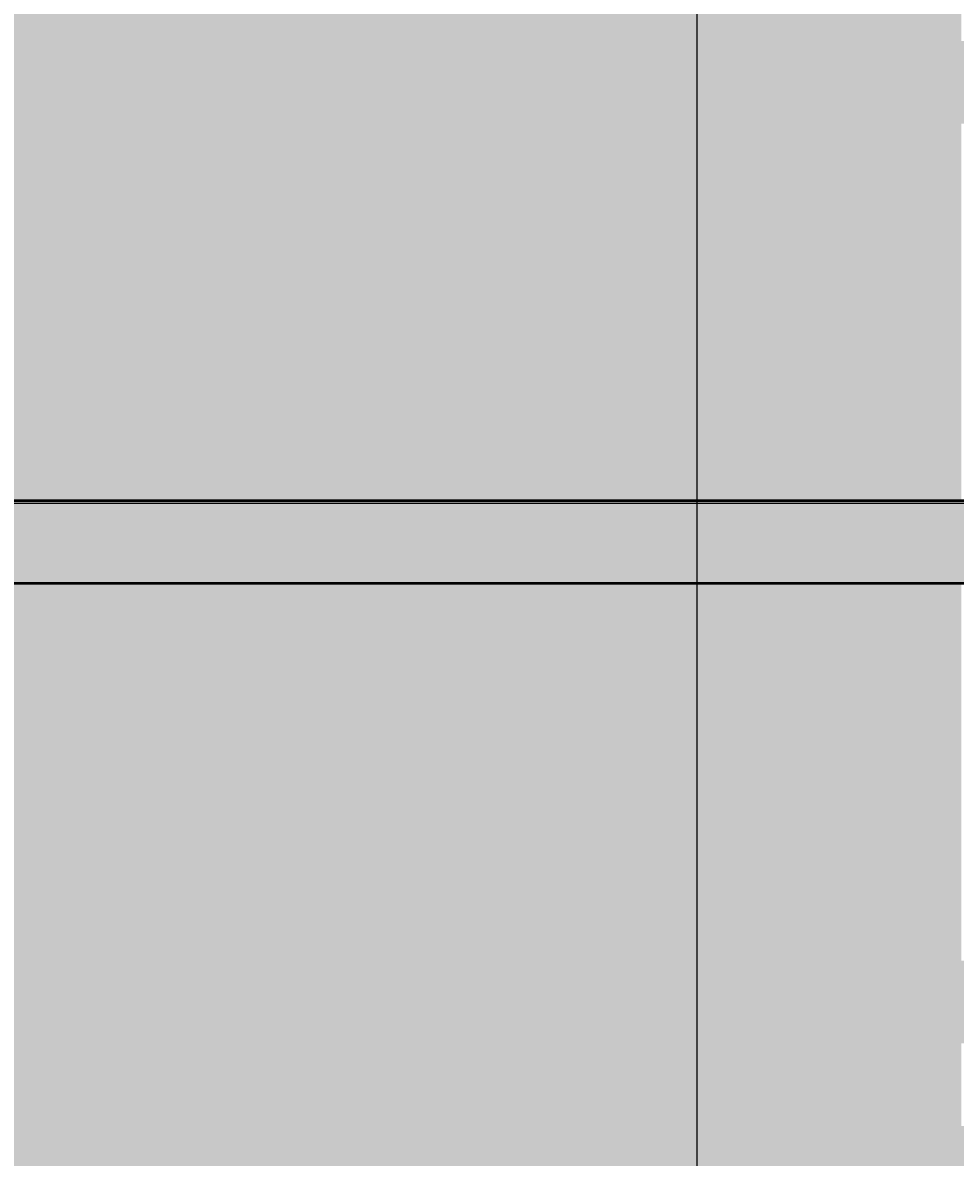
# Model space of a CAD drawing. Units: inches. Extents: x -12 to 334, y -10 to 186.
# Tile 15 of 77: x 42 to 64, y 65 to 92. Entities that reach past the tile are written whole.
import ezdxf

# ---------------------------------------------------------------- set-up
doc = ezdxf.new("R2010")
doc.units = ezdxf.units.IN
doc.header["$MEASUREMENT"] = 0
for name, color, linetype, lineweight in [('M-DIMS', 2, 'Continuous', 18), ('M-EQPM', 7, 'Continuous', 50), ('M-EQPM-PATT', 8, 'Continuous', 18)]:
    doc.layers.add(name, color=color, linetype=linetype, lineweight=lineweight)
doc.styles.get("Standard").update_dxf_attribs({"font": 'arial.ttf'})
doc.dimstyles.get("Standard").update_dxf_attribs({"dimtxt": 0.18, "dimasz": 0.18, "dimexe": 0.18, "dimexo": 0.0625, "dimgap": 0.09, "dimtad": 0, "dimtih": 1, "dimtoh": 1, "dimdec": 4, "dimzin": 0, "dimdsep": 46, "dimtxsty": 'Standard', "dimcen": 0.09, "dimadec": 0, "dimazin": 0, "dimtfac": 1, "dimtdec": 4, "dimtofl": 0, "dimtmove": 0, "dimatfit": 3, "dimfxl": 1, "dimtolj": 1, "dimtzin": 0, "dimarcsym": 0})

# ---------------------------------------------------------------- blocks, each defined once
blk = doc.blocks.new('*D1')
at = {"layer": 'Defpoints', "color": 0, "transparency": 16777216}
for p in [(281.426, 91.899), (3.376, 80.692), (281.426, 14.304)]:
    blk.add_point(p, dxfattribs=at)
at = {"layer": 'M-DIMS', "color": 0, "lineweight": -2, "transparency": 16777216}
for p, q in [((281.426, 91.836), (281.426, 14.124)), ((3.376, 80.629), (3.376, 14.124)), ((3.556, 14.304), (141.935, 14.304)), ((281.246, 14.304), (142.867, 14.304))]:
    blk.add_line(p, q, dxfattribs=at)
at = {"layer": 'M-DIMS', "color": 0, "transparency": 16777216}
for points in [[(3.556, 14.334), (3.556, 14.274), (3.376, 14.304)], [(281.246, 14.334), (281.246, 14.274), (281.426, 14.304)]]:
    blk.add_solid(points, dxfattribs=at)
at = {"layer": 'M-DIMS', "color": 0, "transparency": 16777216, "insert": (142.401, 14.304), "char_height": 0.18, "attachment_point": 5}
blk.add_mtext('\\A1;278.05', dxfattribs=at)
blk = doc.blocks.new('*D14')
at = {"layer": 'Defpoints', "color": 0, "transparency": 16777216}
for p in [(63.5, 109.058), (-11.174, 49.45), (64.207, 49.45)]:
    blk.add_point(p, dxfattribs=at)
at = {"layer": 'M-DIMS', "color": 0, "lineweight": -2, "transparency": 16777216}
for p, q in [((63.438, 109.058), (-11.354, 109.058)), ((-11.174, 108.878), (-11.174, 79.436)), ((-11.174, 49.63), (-11.174, 79.072)), ((64.144, 49.45), (-11.354, 49.45))]:
    blk.add_line(p, q, dxfattribs=at)
at = {"layer": 'M-DIMS', "color": 0, "transparency": 16777216}
for points in [[(-11.204, 108.878), (-11.144, 108.878), (-11.174, 109.058)], [(-11.204, 49.63), (-11.144, 49.63), (-11.174, 49.45)]]:
    blk.add_solid(points, dxfattribs=at)
at = {"layer": 'M-DIMS', "color": 0, "transparency": 16777216, "insert": (-11.174, 79.254), "char_height": 0.18, "attachment_point": 5}
blk.add_mtext('\\A1;59.61', dxfattribs=at)
blk = doc.blocks.new('*D26')
at = {"layer": 'Defpoints', "color": 0, "transparency": 16777216}
for p in [(87.888, 169.385), (87.888, 56.321), (58.1, 33.675)]:
    blk.add_point(p, dxfattribs=at)
at = {"layer": 'M-DIMS', "color": 0, "lineweight": -2, "transparency": 16777216}
for p, q in [((58.1, 33.738), (58.1, 169.565)), ((58.28, 169.385), (72.599, 169.385)), ((87.708, 169.385), (73.389, 169.385)), ((87.888, 56.383), (87.888, 169.565))]:
    blk.add_line(p, q, dxfattribs=at)
at = {"layer": 'M-DIMS', "color": 0, "transparency": 16777216}
for points in [[(58.28, 169.415), (58.28, 169.355), (58.1, 169.385)], [(87.708, 169.415), (87.708, 169.355), (87.888, 169.385)]]:
    blk.add_solid(points, dxfattribs=at)
at = {"layer": 'M-DIMS', "color": 0, "transparency": 16777216, "insert": (72.994, 169.385), "char_height": 0.18, "attachment_point": 5}
blk.add_mtext('\\A1;29.79', dxfattribs=at)
blk = doc.blocks.new('*D35')
at = {"layer": 'Defpoints', "color": 0, "transparency": 16777216}
for p in [(216.428, 98.108), (-11.174, 61.105), (216.428, 61.105)]:
    blk.add_point(p, dxfattribs=at)
at = {"layer": 'M-DIMS', "color": 0, "lineweight": -2, "transparency": 16777216}
for p, q in [((216.365, 98.108), (-11.354, 98.108)), ((-11.174, 97.928), (-11.174, 79.788)), ((-11.174, 61.285), (-11.174, 79.424)), ((216.365, 61.105), (-11.354, 61.105))]:
    blk.add_line(p, q, dxfattribs=at)
at = {"layer": 'M-DIMS', "color": 0, "transparency": 16777216}
for points in [[(-11.204, 97.928), (-11.144, 97.928), (-11.174, 98.108)], [(-11.204, 61.285), (-11.144, 61.285), (-11.174, 61.105)]]:
    blk.add_solid(points, dxfattribs=at)
at = {"layer": 'M-DIMS', "color": 0, "transparency": 16777216, "insert": (-11.174, 79.606), "char_height": 0.18, "attachment_point": 5}
blk.add_mtext('\\A1;37', dxfattribs=at)
blk = doc.blocks.new('*D39')
at = {"layer": 'Defpoints', "color": 0, "transparency": 16777216}
for p in [(279.726, 80.692), (-11.174, 45.854), (269.381, 45.854)]:
    blk.add_point(p, dxfattribs=at)
at = {"layer": 'M-DIMS', "color": 0, "lineweight": -2, "transparency": 16777216}
for p, q in [((279.664, 80.692), (-11.354, 80.692)), ((-11.174, 80.512), (-11.174, 63.455)), ((-11.174, 46.034), (-11.174, 63.091)), ((269.318, 45.854), (-11.354, 45.854))]:
    blk.add_line(p, q, dxfattribs=at)
at = {"layer": 'M-DIMS', "color": 0, "transparency": 16777216}
for points in [[(-11.204, 80.512), (-11.144, 80.512), (-11.174, 80.692)], [(-11.204, 46.034), (-11.144, 46.034), (-11.174, 45.854)]]:
    blk.add_solid(points, dxfattribs=at)
at = {"layer": 'M-DIMS', "color": 0, "transparency": 16777216, "insert": (-11.174, 63.273), "char_height": 0.18, "attachment_point": 5}
blk.add_mtext('\\A1;34.84', dxfattribs=at)

msp = doc.modelspace()

# ---------------------------------------------------------------- hatches: boundary and pattern name
at = {"layer": 'M-EQPM-PATT'}
h = msp.add_hatch(color=256, dxfattribs=at)
h.set_gradient(color1=(99, 100, 102), color2=(99, 100, 102), tint=1)
h.paths.add_polyline_path([(4.3766, 80.754, -0.4132606), (23.5807, 99.8958), (37.1002, 99.8958), (37.1002, 127.7078), (32.1002, 127.7078), (32.1002, 125.2078), (36.1002, 125.2078), (36.1002, 100.8958), (23.5807, 100.8958, 1), (23.5807, 60.4872), (36.1002, 60.4872), (36.1002, 36.1752), (32.1002, 36.1752), (32.1002, 33.6752), (37.1002, 33.6752), (37.1002, 61.4872), (23.5807, 61.4872, -0.384914), (4.4744, 78.754), (72.9244, 78.754), (72.9244, 69.6117), (75.9244, 69.6117), (75.9244, 89.8963), (72.9244, 89.8963), (72.9244, 80.754)])
h.paths.add_polyline_path([(54.1002, 125.2078), (58.1002, 125.2078), (58.1002, 127.7078), (53.1002, 127.7078), (53.1002, 99.8958), (64.5, 99.8958), (64.5, 109.0583), (63.5, 109.0583), (63.5, 100.8958), (54.1002, 100.8958)], flags=17)
h.paths.add_polyline_path([(53.1002, 33.6752), (58.1002, 33.6752), (58.1002, 36.1752), (54.1002, 36.1752), (54.1002, 60.4872), (64.2068, 60.4872), (64.2068, 49.4497), (87.8879, 49.4497), (87.8879, 55.3205), (104.8919, 55.3205), (104.8919, 30.8541), (99.8919, 30.8541), (99.8919, 28.8541), (105.8919, 28.8541), (105.8919, 56.3205), (87.8879, 56.3205), (87.8879, 63.6117), (86.8879, 63.6117), (86.8879, 50.4497), (65.0061, 50.4497), (65.0061, 63.6117), (64.5, 63.6117), (64.5, 61.4872), (53.1002, 61.4872)])
h.paths.add_polyline_path([(121.8919, 28.8541), (121.8919, 30.8541), (116.8919, 30.8541), (116.8919, 45.8541), (209.6965, 45.8541), (209.9204, 46.8541), (115.8919, 46.8541), (115.8919, 28.8541)])
h.paths.add_polyline_path([(221.5761, 32.8541), (216.5761, 32.8541), (216.5761, 30.8541), (222.5761, 30.8541), (222.5761, 46.8541), (209.9204, 46.8541), (209.6965, 45.8541), (221.5761, 45.8541)])
h.paths.add_polyline_path([(233.5761, 45.8541), (249.8485, 45.8541), (249.3759, 46.8541), (232.5761, 46.8541), (232.5761, 30.8541), (238.5761, 30.8541), (238.5761, 32.8541), (233.5761, 32.8541)])
h = msp.add_hatch(color=256, dxfattribs=at)
h.set_gradient(color1=(205, 32, 39), color2=(205, 32, 39), tint=1)
h.paths.add_polyline_path([(64.5, 80.754), (64.5, 89.8963), (226.6083, 89.8963, -1), (226.6083, 69.6117), (64.5, 69.6117), (64.5, 78.754), (4.4744, 78.754, 0.384914), (23.5807, 61.4872), (37.1002, 61.4872), (37.1002, 33.6752), (53.1002, 33.6752), (53.1002, 61.4872), (64.5, 61.4872), (64.5, 63.6117), (226.6083, 63.6117, 1), (226.6083, 95.8963), (64.5, 95.8963), (64.5, 99.8958), (53.1002, 99.8958), (53.1002, 127.7078), (37.1002, 127.7078), (37.1002, 99.8958), (23.5807, 99.8958, 0.4132606), (4.3766, 80.754)])
h.paths.add_polyline_path([(64.5, 91.8963), (64.5, 93.8963), (226.6083, 93.8963, -1), (226.6083, 65.6117), (64.5, 65.6117), (64.5, 67.6117), (226.6083, 67.6117, 1), (226.6083, 91.8963)], flags=16)

# ---------------------------------------------------------------- linework, layer by layer
at = {"layer": 'M-EQPM'}
for p, q in [((72.9244, 80.754), (4.3766, 80.754)), ((72.9244, 78.754), (4.4744, 78.754))]:
    msp.add_line(p, q, dxfattribs=at)

# ---------------------------------------------------------------- dimensions: what is measured, and where the dimension line sits
at = {"layer": 'M-DIMS'}
for base, p1, p2, picture, middle in [((87.8879, 169.3845), (58.1002, 33.6752), (87.8879, 56.3205), '*D26', (72.9941, 169.3845)), ((281.4256, 14.3041), (3.3765, 80.6915), (281.4256, 91.8988), '*D1', (142.401, 14.3041))]:
    dim = msp.add_linear_dim(base=base, p1=p1, p2=p2, dimstyle='Standard', override={"dimdec": 2, "dimlfac": 1, "dimrnd": 0, "dimzin": 0, "dimdsep": 46, "dimlunit": 2}, dxfattribs=at)
    dim.commit()
    dim.dimension.update_dxf_attribs({"geometry": picture, "text_midpoint": middle})
for base, p1, p2, override, picture, middle in [((-11.1736, 49.4497), (63.5, 109.0583), (64.2068, 49.4497), {"dimdec": 2, "dimlfac": 1, "dimrnd": 0, "dimzin": 0, "dimdsep": 46, "dimlunit": 2}, '*D14', (-11.1735, 79.254)), ((-11.1736, 61.1045), (216.4278, 98.1081), (216.4278, 61.1045), {"dimdec": 0, "dimlfac": 1, "dimrnd": 0, "dimzin": 0, "dimdsep": 46, "dimlunit": 2}, '*D35', (-11.1735, 79.6063)), ((-11.1736, 45.8541), (279.7263, 80.6915), (269.3808, 45.8541), {"dimdec": 2, "dimlfac": 1, "dimrnd": 0, "dimzin": 0, "dimdsep": 46, "dimlunit": 2}, '*D39', (-11.1735, 63.2728))]:
    dim = msp.add_linear_dim(base=base, p1=p1, p2=p2, angle=90, dimstyle='Standard', override=override, dxfattribs=at)
    dim.commit()
    dim.dimension.update_dxf_attribs({"geometry": picture, "text_midpoint": middle})

doc.saveas('drawing.dxf')
